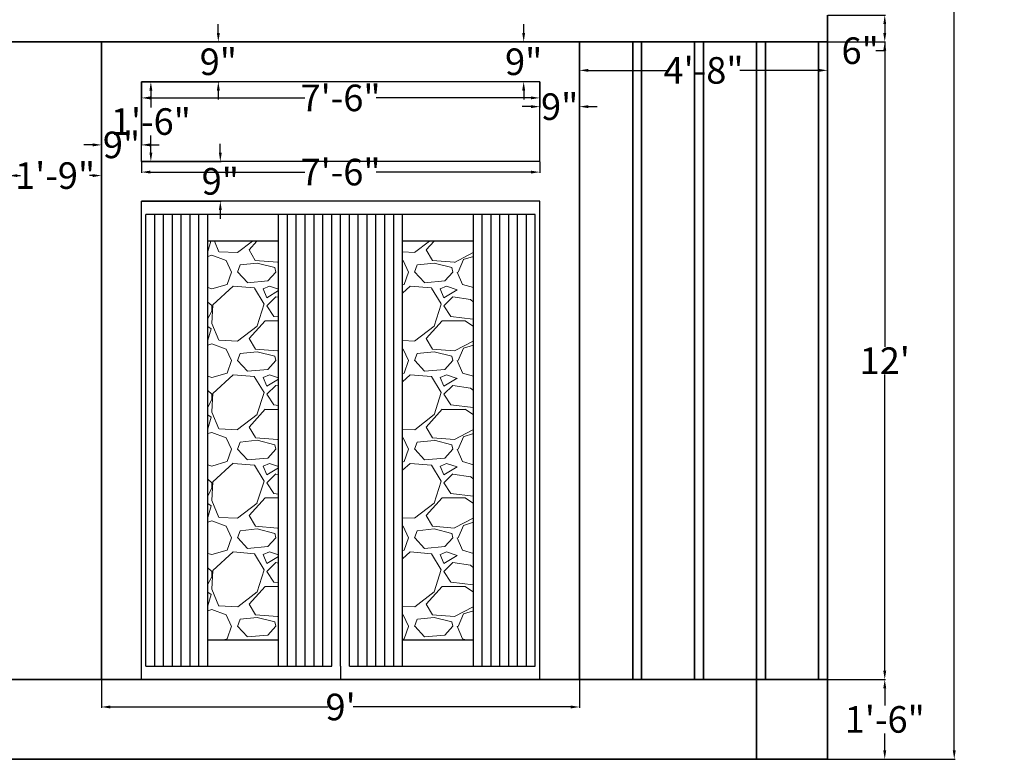
# Model space of a CAD drawing. Units: inches. Extents: x 786 to 1239, y 110 to 563.
# Tile 2 of 3: x 1017 to 1239, y 110 to 277. Entities that reach past the tile are written whole.
import ezdxf

# ---------------------------------------------------------------- set-up
doc = ezdxf.new("R2010")
doc.units = ezdxf.units.IN
doc.header["$MEASUREMENT"] = 0
for name, color, linetype, lineweight in [('A-ANNO-DIMS', 2, 'Continuous', 18), ('A-DOOR', 4, 'Continuous', 25), ('A-ELEV', 7, 'Continuous', 35), ('A-ELEV-PATT', 8, 'Continuous', 13)]:
    doc.layers.add(name, color=color, linetype=linetype, lineweight=lineweight)
doc.styles.get("Standard").update_dxf_attribs({"font": 'arial.ttf'})
doc.dimstyles.get("Standard").update_dxf_attribs({"dimtxt": 6, "dimasz": 2, "dimexe": 0.18, "dimexo": 0.0625, "dimgap": 0.09, "dimtad": 0, "dimtih": 1, "dimtoh": 1, "dimdec": 1, "dimzin": 0, "dimdsep": 46, "dimlunit": 4, "dimtxsty": 'Standard', "dimcen": 0.09, "dimadec": 0, "dimazin": 0, "dimtfac": 1, "dimtdec": 1, "dimtofl": 0, "dimtmove": 0, "dimatfit": 3, "dimfxl": 1, "dimtolj": 1, "dimtzin": 0, "dimarcsym": 0})

# ---------------------------------------------------------------- blocks, each defined once
blk = doc.blocks.new('*D1')
at = {"layer": 'A-ANNO-DIMS', "color": 0, "lineweight": -2, "transparency": 16777216}
for p, q in [((1044.19, 245.05), (1044.19, 242.52)), ((1134.19, 245.05), (1134.19, 242.52)), ((1046.19, 242.7), (1081.15, 242.7)), ((1132.19, 242.7), (1097.23, 242.7))]:
    blk.add_line(p, q, dxfattribs=at)
at = {"layer": 'A-ANNO-DIMS', "color": 0, "transparency": 16777216}
for points in [[(1046.19, 243.03), (1046.19, 242.37), (1044.19, 242.7)], [(1132.19, 243.03), (1132.19, 242.37), (1134.19, 242.7)]]:
    blk.add_solid(points, dxfattribs=at)
at = {"layer": 'Defpoints', "color": 0, "transparency": 16777216}
for p in [(1044.19, 245.11), (1134.19, 245.11), (1044.19, 242.7)]:
    blk.add_point(p, dxfattribs=at)
at = {"layer": 'A-ANNO-DIMS', "color": 0, "transparency": 16777216, "insert": (1089.19, 242.7), "char_height": 6, "attachment_point": 5}
blk.add_mtext('\\A1;7\'-6"', dxfattribs=at)
blk = doc.blocks.new('*D2')
at = {"layer": 'A-ANNO-DIMS', "color": 0, "lineweight": -2, "transparency": 16777216}
for p, q in [((1044.26, 263.11), (1046.51, 263.11)), ((1046.33, 261.11), (1046.33, 257.26)), ((1046.33, 247.11), (1046.33, 250.96)), ((1044.26, 245.11), (1046.51, 245.11))]:
    blk.add_line(p, q, dxfattribs=at)
at = {"layer": 'A-ANNO-DIMS', "color": 0, "transparency": 16777216}
for points in [[(1046, 261.11), (1046.66, 261.11), (1046.33, 263.11)], [(1046, 247.11), (1046.66, 247.11), (1046.33, 245.11)]]:
    blk.add_solid(points, dxfattribs=at)
at = {"layer": 'Defpoints', "color": 0, "transparency": 16777216}
for p in [(1044.19, 263.11), (1046.33, 263.11), (1044.19, 245.11)]:
    blk.add_point(p, dxfattribs=at)
at = {"layer": 'A-ANNO-DIMS', "color": 0, "transparency": 16777216, "insert": (1046.33, 254.11), "char_height": 6, "attachment_point": 5}
blk.add_mtext('\\A1;1\'-6"', dxfattribs=at)
blk = doc.blocks.new('*D3')
at = {"layer": 'A-ANNO-DIMS', "color": 0, "lineweight": -2, "transparency": 16777216}
for p, q in [((1130.56, 274.11), (1130.56, 276.11)), ((1143.13, 272.11), (1130.38, 272.11)), ((1134.13, 263.11), (1130.38, 263.11)), ((1130.56, 261.11), (1130.56, 259.11))]:
    blk.add_line(p, q, dxfattribs=at)
at = {"layer": 'A-ANNO-DIMS', "color": 0, "transparency": 16777216}
for points in [[(1130.23, 274.11), (1130.89, 274.11), (1130.56, 272.11)], [(1130.23, 261.11), (1130.89, 261.11), (1130.56, 263.11)]]:
    blk.add_solid(points, dxfattribs=at)
at = {"layer": 'Defpoints', "color": 0, "transparency": 16777216}
for p in [(1130.56, 272.11), (1143.19, 272.11), (1134.19, 263.11)]:
    blk.add_point(p, dxfattribs=at)
at = {"layer": 'A-ANNO-DIMS', "color": 0, "transparency": 16777216, "insert": (1130.56, 267.61), "char_height": 6, "attachment_point": 5}
blk.add_mtext('\\A1;9"', dxfattribs=at)
blk = doc.blocks.new('*D4')
at = {"layer": 'A-ANNO-DIMS', "color": 0, "lineweight": -2, "transparency": 16777216}
for p, q in [((1143.19, 272.05), (1143.19, 257.3)), ((1134.19, 263.05), (1134.19, 257.3)), ((1132.19, 257.48), (1130.19, 257.48)), ((1145.19, 257.48), (1147.19, 257.48))]:
    blk.add_line(p, q, dxfattribs=at)
at = {"layer": 'A-ANNO-DIMS', "color": 0, "transparency": 16777216}
for points in [[(1132.19, 257.81), (1132.19, 257.14), (1134.19, 257.48)], [(1145.19, 257.81), (1145.19, 257.14), (1143.19, 257.48)]]:
    blk.add_solid(points, dxfattribs=at)
at = {"layer": 'Defpoints', "color": 0, "transparency": 16777216}
for p in [(1143.19, 272.11), (1134.19, 263.11), (1143.19, 257.48)]:
    blk.add_point(p, dxfattribs=at)
at = {"layer": 'A-ANNO-DIMS', "color": 0, "transparency": 16777216, "insert": (1138.69, 257.48), "char_height": 6, "attachment_point": 5}
blk.add_mtext('\\A1;9"', dxfattribs=at)
blk = doc.blocks.new('*D5')
at = {"layer": 'A-ANNO-DIMS', "color": 0, "lineweight": -2, "transparency": 16777216}
for p, q in [((1062.02, 247.11), (1062.02, 249.11)), ((1044.26, 245.11), (1062.2, 245.11)), ((1044.26, 236.11), (1062.2, 236.11)), ((1062.02, 234.11), (1062.02, 232.11))]:
    blk.add_line(p, q, dxfattribs=at)
at = {"layer": 'A-ANNO-DIMS', "color": 0, "transparency": 16777216}
for points in [[(1061.69, 247.11), (1062.36, 247.11), (1062.02, 245.11)], [(1061.69, 234.11), (1062.36, 234.11), (1062.02, 236.11)]]:
    blk.add_solid(points, dxfattribs=at)
at = {"layer": 'Defpoints', "color": 0, "transparency": 16777216}
for p in [(1044.19, 245.11), (1044.19, 236.11), (1062.02, 236.11)]:
    blk.add_point(p, dxfattribs=at)
at = {"layer": 'A-ANNO-DIMS', "color": 0, "transparency": 16777216, "insert": (1062.02, 240.61), "char_height": 6, "attachment_point": 5}
blk.add_mtext('\\A1;9"', dxfattribs=at)
blk = doc.blocks.new('*D6')
at = {"layer": 'A-ANNO-DIMS', "color": 0, "lineweight": -2, "transparency": 16777216}
for p, q in [((1035.19, 272.05), (1035.19, 248.66)), ((1044.19, 263.05), (1044.19, 248.66)), ((1033.19, 248.84), (1031.19, 248.84)), ((1046.19, 248.84), (1048.19, 248.84))]:
    blk.add_line(p, q, dxfattribs=at)
at = {"layer": 'A-ANNO-DIMS', "color": 0, "transparency": 16777216}
for points in [[(1033.19, 249.18), (1033.19, 248.51), (1035.19, 248.84)], [(1046.19, 249.18), (1046.19, 248.51), (1044.19, 248.84)]]:
    blk.add_solid(points, dxfattribs=at)
at = {"layer": 'Defpoints', "color": 0, "transparency": 16777216}
for p in [(1035.19, 272.11), (1044.19, 263.11), (1044.19, 248.84)]:
    blk.add_point(p, dxfattribs=at)
at = {"layer": 'A-ANNO-DIMS', "color": 0, "transparency": 16777216, "insert": (1039.69, 248.84), "char_height": 6, "attachment_point": 5}
blk.add_mtext('\\A1;9"', dxfattribs=at)
blk = doc.blocks.new('*D7')
at = {"layer": 'A-ANNO-DIMS', "color": 0, "lineweight": -2, "transparency": 16777216}
for p, q in [((1035.19, 272.05), (1035.19, 241.73)), ((1014.19, 245.05), (1014.19, 241.73)), ((1016.19, 241.91), (1016.91, 241.91)), ((1033.19, 241.91), (1032.48, 241.91))]:
    blk.add_line(p, q, dxfattribs=at)
at = {"layer": 'A-ANNO-DIMS', "color": 0, "transparency": 16777216}
for points in [[(1016.19, 242.24), (1016.19, 241.58), (1014.19, 241.91)], [(1033.19, 242.24), (1033.19, 241.58), (1035.19, 241.91)]]:
    blk.add_solid(points, dxfattribs=at)
at = {"layer": 'Defpoints', "color": 0, "transparency": 16777216}
for p in [(1035.19, 272.11), (1014.19, 245.11), (1035.19, 241.91)]:
    blk.add_point(p, dxfattribs=at)
at = {"layer": 'A-ANNO-DIMS', "color": 0, "transparency": 16777216, "insert": (1024.69, 241.91), "char_height": 6, "attachment_point": 5}
blk.add_mtext('\\A1;1\'-9"', dxfattribs=at)
blk = doc.blocks.new('*D9')
at = {"layer": 'A-ANNO-DIMS', "color": 0, "lineweight": -2, "transparency": 16777216}
for p, q in [((1143.19, 272.05), (1143.19, 265.49)), ((1199.19, 272.05), (1199.19, 265.49)), ((1145.19, 265.67), (1163.01, 265.67)), ((1197.19, 265.67), (1179.38, 265.67))]:
    blk.add_line(p, q, dxfattribs=at)
at = {"layer": 'A-ANNO-DIMS', "color": 0, "transparency": 16777216}
for points in [[(1145.19, 266), (1145.19, 265.33), (1143.19, 265.67)], [(1197.19, 266), (1197.19, 265.33), (1199.19, 265.67)]]:
    blk.add_solid(points, dxfattribs=at)
at = {"layer": 'Defpoints', "color": 0, "transparency": 16777216}
for p in [(1143.19, 272.11), (1199.19, 272.11), (1199.19, 265.67)]:
    blk.add_point(p, dxfattribs=at)
at = {"layer": 'A-ANNO-DIMS', "color": 0, "transparency": 16777216, "insert": (1171.19, 265.67), "char_height": 6, "attachment_point": 5}
blk.add_mtext('\\A1;4\'-8"', dxfattribs=at)
blk = doc.blocks.new('*D33')
at = {"layer": 'A-ANNO-DIMS', "color": 0, "lineweight": -2, "transparency": 16777216}
for p, q in [((1035.19, 128.05), (1035.19, 121.74)), ((1143.19, 128.05), (1143.19, 121.74)), ((1037.19, 121.92), (1086.34, 121.92)), ((1141.19, 121.92), (1092.04, 121.92))]:
    blk.add_line(p, q, dxfattribs=at)
at = {"layer": 'A-ANNO-DIMS', "color": 0, "transparency": 16777216}
for points in [[(1037.19, 122.26), (1037.19, 121.59), (1035.19, 121.92)], [(1141.19, 122.26), (1141.19, 121.59), (1143.19, 121.92)]]:
    blk.add_solid(points, dxfattribs=at)
at = {"layer": 'Defpoints', "color": 0, "transparency": 16777216}
for p in [(1035.19, 128.11), (1143.19, 128.11), (1143.19, 121.92)]:
    blk.add_point(p, dxfattribs=at)
at = {"layer": 'A-ANNO-DIMS', "color": 0, "transparency": 16777216, "insert": (1089.19, 121.92), "char_height": 6, "attachment_point": 5}
blk.add_mtext("\\A1;9'", dxfattribs=at)
blk = doc.blocks.new('*D34')
at = {"layer": 'A-ANNO-DIMS', "color": 0, "lineweight": -2, "transparency": 16777216}
for p, q in [((1199.26, 128.11), (1212.32, 128.11)), ((1212.14, 126.11), (1212.14, 122.26)), ((1212.14, 112.11), (1212.14, 115.96)), ((1199.26, 110.11), (1212.32, 110.11))]:
    blk.add_line(p, q, dxfattribs=at)
at = {"layer": 'A-ANNO-DIMS', "color": 0, "transparency": 16777216}
for points in [[(1211.81, 126.11), (1212.47, 126.11), (1212.14, 128.11)], [(1211.81, 112.11), (1212.47, 112.11), (1212.14, 110.11)]]:
    blk.add_solid(points, dxfattribs=at)
at = {"layer": 'Defpoints', "color": 0, "transparency": 16777216}
for p in [(1199.19, 128.11), (1199.19, 110.11), (1212.14, 110.11)]:
    blk.add_point(p, dxfattribs=at)
at = {"layer": 'A-ANNO-DIMS', "color": 0, "transparency": 16777216, "insert": (1212.14, 119.11), "char_height": 6, "attachment_point": 5}
blk.add_mtext('\\A1;1\'-6"', dxfattribs=at)
blk = doc.blocks.new('*D35')
at = {"layer": 'A-ANNO-DIMS', "color": 0, "lineweight": -2, "transparency": 16777216}
for p, q in [((1199.26, 272.11), (1212.32, 272.11)), ((1212.14, 270.11), (1212.14, 203.21)), ((1212.14, 130.11), (1212.14, 197.01)), ((1199.26, 128.11), (1212.32, 128.11))]:
    blk.add_line(p, q, dxfattribs=at)
at = {"layer": 'A-ANNO-DIMS', "color": 0, "transparency": 16777216}
for points in [[(1211.81, 270.11), (1212.47, 270.11), (1212.14, 272.11)], [(1211.81, 130.11), (1212.47, 130.11), (1212.14, 128.11)]]:
    blk.add_solid(points, dxfattribs=at)
at = {"layer": 'Defpoints', "color": 0, "transparency": 16777216}
for p in [(1199.19, 272.11), (1212.14, 272.11), (1199.19, 128.11)]:
    blk.add_point(p, dxfattribs=at)
at = {"layer": 'A-ANNO-DIMS', "color": 0, "transparency": 16777216, "insert": (1212.14, 200.11), "char_height": 6, "attachment_point": 5}
blk.add_mtext("\\A1;12'", dxfattribs=at)
blk = doc.blocks.new('*D36')
at = {"layer": 'A-ANNO-DIMS', "color": 0, "lineweight": -2, "transparency": 16777216}
for p, q in [((1199.26, 278.11), (1212.32, 278.11)), ((1212.14, 276.11), (1212.14, 274.11)), ((1199.26, 272.11), (1212.32, 272.11)), ((1212.14, 272.11), (1212.14, 270.11)), ((1212.14, 270.11), (1210.14, 270.11))]:
    blk.add_line(p, q, dxfattribs=at)
at = {"layer": 'A-ANNO-DIMS', "color": 0, "transparency": 16777216}
for points in [[(1211.81, 276.11), (1212.47, 276.11), (1212.14, 278.11)], [(1211.81, 274.11), (1212.47, 274.11), (1212.14, 272.11)]]:
    blk.add_solid(points, dxfattribs=at)
at = {"layer": 'Defpoints', "color": 0, "transparency": 16777216}
for p in [(1199.19, 278.11), (1199.19, 272.11), (1212.14, 272.11)]:
    blk.add_point(p, dxfattribs=at)
at = {"layer": 'A-ANNO-DIMS', "color": 0, "transparency": 16777216, "insert": (1206.58, 270.11), "char_height": 6, "attachment_point": 5}
blk.add_mtext('\\A1;6"', dxfattribs=at)
blk = doc.blocks.new('*D41')
at = {"layer": 'A-ANNO-DIMS', "color": 0, "lineweight": -2, "transparency": 16777216}
for p, q in [((1044.19, 263.05), (1044.19, 259.27)), ((1134.19, 263.05), (1134.19, 259.27)), ((1046.19, 259.45), (1081.15, 259.45)), ((1132.19, 259.45), (1097.23, 259.45))]:
    blk.add_line(p, q, dxfattribs=at)
at = {"layer": 'A-ANNO-DIMS', "color": 0, "transparency": 16777216}
for points in [[(1046.19, 259.78), (1046.19, 259.12), (1044.19, 259.45)], [(1132.19, 259.78), (1132.19, 259.12), (1134.19, 259.45)]]:
    blk.add_solid(points, dxfattribs=at)
at = {"layer": 'Defpoints', "color": 0, "transparency": 16777216}
for p in [(1044.19, 263.11), (1134.19, 263.11), (1044.19, 259.45)]:
    blk.add_point(p, dxfattribs=at)
at = {"layer": 'A-ANNO-DIMS', "color": 0, "transparency": 16777216, "insert": (1089.19, 259.45), "char_height": 6, "attachment_point": 5}
blk.add_mtext('\\A1;7\'-6"', dxfattribs=at)
blk = doc.blocks.new('*D42')
at = {"layer": 'A-ANNO-DIMS', "color": 0, "lineweight": -2, "transparency": 16777216}
for p, q in [((1061.57, 274.11), (1061.57, 276.11)), ((1035.26, 272.11), (1061.75, 272.11)), ((1044.26, 263.11), (1061.75, 263.11)), ((1061.57, 261.11), (1061.57, 259.11))]:
    blk.add_line(p, q, dxfattribs=at)
at = {"layer": 'A-ANNO-DIMS', "color": 0, "transparency": 16777216}
for points in [[(1061.24, 274.11), (1061.91, 274.11), (1061.57, 272.11)], [(1061.24, 261.11), (1061.91, 261.11), (1061.57, 263.11)]]:
    blk.add_solid(points, dxfattribs=at)
at = {"layer": 'Defpoints', "color": 0, "transparency": 16777216}
for p in [(1035.19, 272.11), (1044.19, 263.11), (1061.57, 263.11)]:
    blk.add_point(p, dxfattribs=at)
at = {"layer": 'A-ANNO-DIMS', "color": 0, "transparency": 16777216, "insert": (1061.57, 267.61), "char_height": 6, "attachment_point": 5}
blk.add_mtext('\\A1;9"', dxfattribs=at)
blk = doc.blocks.new('*D48')
at = {"layer": 'A-ANNO-DIMS', "color": 0, "lineweight": -2, "transparency": 16777216}
for p, q in [((1205.26, 544.11), (1228.02, 544.11)), ((1227.84, 542.11), (1227.84, 330.26)), ((1227.84, 112.11), (1227.84, 323.95)), ((1199.26, 110.11), (1228.02, 110.11))]:
    blk.add_line(p, q, dxfattribs=at)
at = {"layer": 'A-ANNO-DIMS', "color": 0, "transparency": 16777216}
for points in [[(1227.51, 542.11), (1228.17, 542.11), (1227.84, 544.11)], [(1227.51, 112.11), (1228.17, 112.11), (1227.84, 110.11)]]:
    blk.add_solid(points, dxfattribs=at)
at = {"layer": 'Defpoints', "color": 0, "transparency": 16777216}
for p in [(1205.19, 544.11), (1199.19, 110.11), (1227.84, 110.11)]:
    blk.add_point(p, dxfattribs=at)
at = {"layer": 'A-ANNO-DIMS', "color": 0, "transparency": 16777216, "insert": (1227.84, 327.11), "char_height": 6, "attachment_point": 5}
blk.add_mtext('\\A1;36\'-2"', dxfattribs=at)

msp = doc.modelspace()

# ---------------------------------------------------------------- hatches: boundary and pattern name
at = {"layer": 'A-ELEV-PATT'}
h = msp.add_hatch(dxfattribs=at)
h.set_pattern_fill('GRAVEL', color=256, scale=20)
h.set_pattern_definition([(228.01279, (14.4, 20), (-160, -180), [2.69072, -266.38176]), (184.96974, (12.6, 18), (240, 20), [4.61736, -457.1185]), (132.51045, (8, 17.6), (200, -220), [3.25576, -322.32065]), (267.27369, (0.2, 12.6), (20, 400), [4.20476, -416.27116]), (292.83365, (0, 8.4), (-100, 240), [4.1231, -408.18746]), (357.27369, (1.6, 4.6), (-400, 20), [4.20476, -416.27116]), (37.69424, (5.8, 4.4), (-260, -200), [5.56058, -550.49697]), (72.25533, (10.2, 7.8), (140, 440), [5.24976, -519.72643]), (121.42957, (11.8, 12.8), (-160, 260), [4.219, -417.68146]), (175.23636, (9.6, 16.4), (220, -20), [4.81664, -236.01525]), (222.39744, (4.8, 16.8), (-240, -220), [6.22896, -616.6675]), (138.81407, (20, 12.4), (-140, 120), [2.12602, -210.4769]), (171.46923, (18.4, 13.8), (260, -40), [4.04474, -400.43023]), (225, (14.4, 14.4), (-2e-15, -20), [2.82842, -25.45585]), (203.1986, (13, 16.8), (100, 40), [1.52316, -150.7923]), (291.8014, (11.6, 16.2), (-20, 60), [2.15406, -105.54924]), (30.96376, (12.4, 14.2), (60, 40), [3.49858, -113.12046]), (161.56505, (15.4, 16), (40, -20), [2.52982, -60.71573]), (16.38954, (0, 16.2), (200, 60), [3.544, -350.8569]), (70.34618, (3.4, 17.2), (-80, -220), [2.97322, -294.34815]), (293.1986, (15.4, 20), (-40, 100), [3.0463, -149.26916]), (343.61046, (16.6, 17.2), (-200, 60), [3.544, -350.8569]), (339.44395, (0, 3.8), (-100, 40), [3.4176, -167.46247]), (294.77514, (3.2, 2.6), (-100, 220), [2.86356, -283.49286]), (66.8014, (15.6, 0), (40, 100), [3.0463, -149.26916]), (17.35402, (16.8, 2.8), (-260, -80), [3.35262, -331.90847]), (69.44395, (5.8, 0), (-40, -100), [1.7088, -169.17127]), (101.30993, (14.4, 0), (-20, 80), [1.0198, -100.9606]), (165.96376, (14.2, 1), (60, -20), [4.1231, -78.339]), (186.00901, (10.2, 2), (200, 20), [3.821, -378.27846]), (303.69007, (12.4, 12.4), (-20, 40), [2.88444, -69.2266]), (353.15723, (14, 10), (340, -40), [5.03588, -498.55125]), (60.9454, (19, 9.4), (-80, -140), [2.05912, -203.85348]), (90, (20, 11.2), (-20, 20), [1.2, -18.8]), (120.25644, (9.8, 2.6), (80, -140), [2.77848, -275.0704]), (48.01279, (8.4, 5), (160, 180), [5.38144, -263.69104]), (0, (12, 9), (20, 20), [5.2, -14.8]), (325.30485, (17.2, 9), (200, -140), [3.16228, -313.06549]), (254.0546, (19.8, 7.2), (-20, -80), [2.91204, -142.69016]), (207.645975, (19, 4.4), (-380, -200), [4.7413, -469.38948]), (175.42608, (14.8, 2.2), (-260, 20), [5.01598, -496.58147])])
h.paths.add_polyline_path([(1075.19, 227.11), (1059.19, 227.11), (1059.19, 137.11), (1075.19, 137.11)])
h.paths.add_polyline_path([(1119.19, 227.11), (1103.19, 227.11), (1103.19, 137.11), (1119.19, 137.11)])

# ---------------------------------------------------------------- linework, layer by layer
at = {"layer": 'A-DOOR'}
for p, q in [((1134.19, 263.11), (1044.19, 263.11)), ((1044.19, 245.11), (1044.19, 263.11)), ((1134.19, 245.11), (1134.19, 263.11)), ((1134.19, 245.11), (1044.19, 245.11)), ((1044.19, 128.11), (1044.19, 236.11)), ((1134.19, 236.11), (1044.19, 236.11)), ((1134.19, 128.11), (1134.19, 236.11)), ((1133.19, 233.11), (1045.19, 233.11)), ((1045.19, 131.11), (1045.19, 233.11)), ((1047.19, 131.11), (1047.19, 233.11)), ((1049.19, 131.11), (1049.19, 233.11)), ((1051.19, 131.11), (1051.19, 233.11)), ((1053.19, 131.11), (1053.19, 233.11)), ((1055.19, 131.11), (1055.19, 233.11)), ((1057.19, 131.11), (1057.19, 233.11)), ((1057.19, 131.11), (1057.19, 233.11)), ((1059.19, 131.11), (1059.19, 233.11)), ((1075.19, 131.11), (1075.19, 233.11)), ((1077.19, 131.11), (1077.19, 233.11)), ((1079.19, 131.11), (1079.19, 233.11)), ((1081.19, 131.11), (1081.19, 233.11)), ((1083.19, 131.11), (1083.19, 233.11)), ((1085.19, 131.11), (1085.19, 233.11)), ((1087.19, 131.11), (1087.19, 233.11)), ((1089.19, 131.11), (1089.19, 233.11)), ((1091.19, 131.11), (1091.19, 233.11)), ((1093.19, 131.11), (1093.19, 233.11)), ((1095.19, 131.11), (1095.19, 233.11)), ((1097.19, 131.11), (1097.19, 233.11)), ((1099.19, 131.11), (1099.19, 233.11)), ((1101.19, 131.11), (1101.19, 233.11)), ((1103.19, 131.11), (1103.19, 233.11)), ((1119.19, 131.11), (1119.19, 233.11)), ((1121.19, 131.11), (1121.19, 233.11)), ((1123.19, 131.11), (1123.19, 233.11)), ((1125.19, 131.11), (1125.19, 233.11)), ((1127.19, 131.11), (1127.19, 233.11)), ((1129.19, 131.11), (1129.19, 233.11)), ((1131.19, 131.11), (1131.19, 233.11)), ((1131.19, 131.11), (1131.19, 233.11)), ((1133.19, 131.11), (1133.19, 233.11)), ((1075.19, 227.11), (1059.19, 227.11)), ((1119.19, 227.11), (1103.19, 227.11)), ((1059.19, 137.11), (1075.19, 137.11)), ((1103.19, 137.11), (1119.19, 137.11)), ((1045.19, 131.11), (1087.19, 131.11)), ((1089.19, 131.11), (1089.19, 128.11)), ((1091.19, 131.11), (1133.19, 131.11))]:
    msp.add_line(p, q, dxfattribs=at)
at = {"layer": 'A-ELEV'}
for p, q in [((1199.19, 272.11), (1199.19, 278.11)), ((1199.19, 272.11), (815.19, 272.11)), ((1035.19, 128.11), (1035.19, 272.11)), ((1143.19, 128.11), (1143.19, 272.11)), ((1155.19, 128.11), (1155.19, 272.11)), ((1157.19, 128.11), (1157.19, 272.11)), ((1169.19, 128.11), (1169.19, 272.11)), ((1171.19, 128.11), (1171.19, 272.11)), ((1183.19, 110.11), (1183.19, 272.11)), ((1185.19, 128.11), (1185.19, 272.11)), ((1197.19, 128.11), (1197.19, 272.11)), ((1199.19, 128.11), (1199.19, 272.11)), ((1199.19, 128.11), (815.19, 128.11)), ((1199.19, 110.11), (1199.19, 128.11)), ((815.19, 110.11), (1199.19, 110.11))]:
    msp.add_line(p, q, dxfattribs=at)

# ---------------------------------------------------------------- dimensions: what is measured, and where the dimension line sits
at = {"layer": 'A-ANNO-DIMS'}
for base, p1, p2, picture, middle in [((1227.84, 110.11), (1205.19, 544.11), (1199.19, 110.11), '*D48', (1227.84, 327.11)), ((1212.14, 272.11), (1199.19, 278.11), (1199.19, 272.11), '*D36', (1206.58, 270.11)), ((1061.57, 263.11), (1035.19, 272.11), (1044.19, 263.11), '*D42', (1061.57, 267.61)), ((1130.56, 272.11), (1134.19, 263.11), (1143.19, 272.11), '*D3', (1130.56, 267.61)), ((1212.14, 272.11), (1199.19, 128.11), (1199.19, 272.11), '*D35', (1212.14, 200.11)), ((1046.33, 263.11), (1044.19, 245.11), (1044.19, 263.11), '*D2', (1046.33, 254.11)), ((1062.02, 236.11), (1044.19, 245.11), (1044.19, 236.11), '*D5', (1062.02, 240.61)), ((1212.14, 110.11), (1199.19, 128.11), (1199.19, 110.11), '*D34', (1212.14, 119.11))]:
    dim = msp.add_linear_dim(base=base, p1=p1, p2=p2, angle=90, dimstyle='Standard', override={"dimclrd": 0, "dimclre": 0, "dimclrt": 0}, dxfattribs=at)
    dim.commit()
    dim.dimension.update_dxf_attribs({"geometry": picture, "text_midpoint": middle})
for base, p1, p2, picture, middle in [((1035.19, 241.91), (1014.19, 245.11), (1035.19, 272.11), '*D7', (1024.69, 241.91)), ((1044.19, 248.84), (1035.19, 272.11), (1044.19, 263.11), '*D6', (1039.69, 248.84)), ((1143.19, 257.48), (1134.19, 263.11), (1143.19, 272.11), '*D4', (1138.69, 257.48)), ((1199.19, 265.67), (1143.19, 272.11), (1199.19, 272.11), '*D9', (1171.19, 265.67)), ((1044.19, 259.45), (1134.19, 263.11), (1044.19, 263.11), '*D41', (1089.19, 259.45)), ((1044.19, 242.7), (1134.19, 245.11), (1044.19, 245.11), '*D1', (1089.19, 242.7)), ((1143.19, 121.92), (1035.19, 128.11), (1143.19, 128.11), '*D33', (1089.19, 121.92))]:
    dim = msp.add_linear_dim(base=base, p1=p1, p2=p2, dimstyle='Standard', override={"dimclrd": 0, "dimclre": 0, "dimclrt": 0}, dxfattribs=at)
    dim.commit()
    dim.dimension.update_dxf_attribs({"geometry": picture, "text_midpoint": middle})

doc.saveas('drawing.dxf')
